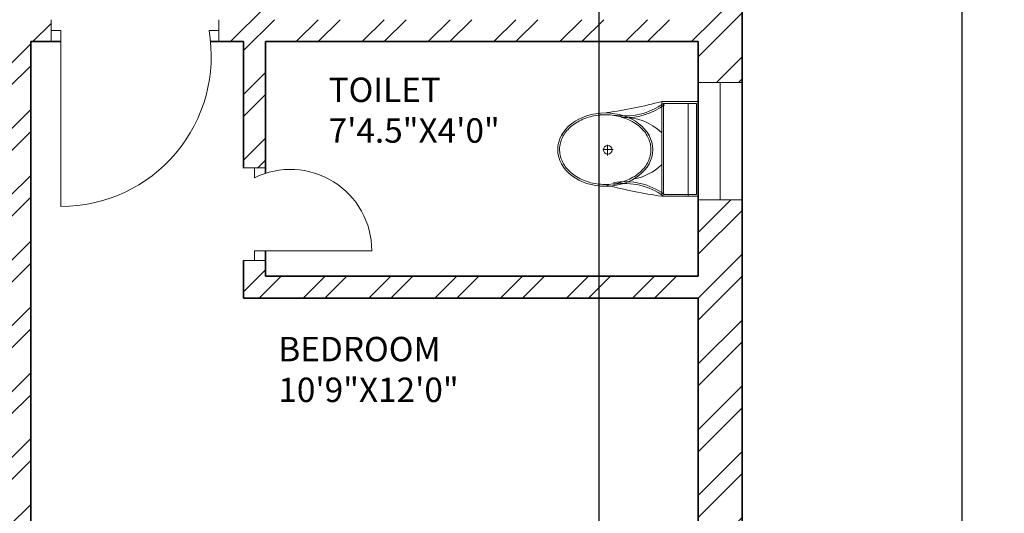
# Model space of a CAD drawing. Units: inches. Extents: x 2120 to 4013, y 1390 to 3019.
# Tile 22 of 59: x 2862 to 3063, y 1690 to 1792. Entities that reach past the tile are written whole.
import ezdxf

# ---------------------------------------------------------------- set-up
doc = ezdxf.new("R2010")
doc.units = ezdxf.units.IN
for name, color, linetype, lineweight in [('A-ANNO-DIMS', 2, 'Continuous', 18), ('A-AREA-IDEN', 7, 'Continuous', 18), ('A-DOOR', 3, 'Continuous', 18), ('A-FLOR-FIXT', 9, 'Continuous', 18), ('A-GLAZ', 4, 'Continuous', 18), ('A-WALL', 7, 'Continuous', 35), ('A-WALL-PATT', 252, 'Continuous', 13)]:
    doc.layers.add(name, color=color, linetype=linetype, lineweight=lineweight)
doc.styles.get("Standard").update_dxf_attribs({"font": 'arial.ttf'})
doc.dimstyles.get("Standard").update_dxf_attribs({"dimtxt": 0.18, "dimasz": 0.18, "dimexe": 0.18, "dimexo": 0.0625, "dimgap": 0.09, "dimtad": 0, "dimtih": 1, "dimtoh": 1, "dimdec": 4, "dimzin": 0, "dimdsep": 46, "dimtxsty": 'Standard', "dimcen": 0.09, "dimadec": 0, "dimazin": 0, "dimtfac": 1, "dimtdec": 4, "dimtofl": 0, "dimtmove": 0, "dimatfit": 3, "dimfxl": 1, "dimtolj": 1, "dimtzin": 0, "dimarcsym": 0})

# ---------------------------------------------------------------- blocks, each defined once
blk = doc.blocks.new('A$C31115884')
for p, q in [((283.1, 497.7), (223.4, 497.7)), ((257.5, 466.4), (257.5, 523.2)), ((0, 200), (0, 0)), ((520, 200), (0, 200)), ((10, 190), (10, 10)), ((510, 190), (10, 190)), ((510, 10), (510, 190)), ((520, 0), (520, 200)), ((510, 54.5), (0, 54.5)), ((10, 10), (510, 10)), ((0, 0), (520, 0))]:
    blk.add_line(p, q)
blk.add_circle((255.6, 496.4), 23.6)
for centre, radius, start, end in [((2777.7, -204.6), 2807, 165.4549, 171.7133), ((3237, 905), 2807, 188.2867, 194.5451), ((-294.5, 403.3), 364.7, 324.2091, 9.3499), ((-294.5, 403.3), 374.7, 324.2091, 9.3499), ((805.8, 403.3), 364.7, 170.6501, 215.7909), ((139.5, 406.2), 293.5, 315.8436, 2.6563), ((805.8, 403.3), 374.7, 179.2036, 215.7909), ((383.6, 406.2), 293.5, 190.2774, 224.1564)]:
    blk.add_arc(centre, radius, start, end)
blk.add_ellipse((256.2, 509.9), major_axis=(0, -260.7), ratio=0.772727)
blk.add_open_spline([(256.2, 259.2), (263.1, 259.2), (270, 259.7), (287.8, 262.3), (298.7, 265.1), (319.9, 273.1), (330.2, 278.4), (350.1, 291.1), (359.7, 298.7), (377.7, 315.9), (386.2, 325.5), (401.7, 346.6), (408.8, 358.1), (421.3, 382.5), (426.8, 395.5), (435.9, 422.4), (439.5, 436.4), (444.8, 465.1), (446.5, 479.7), (447.9, 509.2), (447.6, 524), (445, 553.3), (442.7, 567.8), (436.3, 596), (432.1, 609.7), (421.9, 636), (416, 648.6), (402.5, 672.1), (395, 683), (378.6, 703), (369.8, 712.1), (351.1, 728), (341.3, 734.8), (320.9, 746.2), (310.4, 750.7), (288.9, 757.3), (278, 759.4), (256, 761), (245, 760.6), (223.1, 757.2), (212.3, 754.3), (191.1, 746.1), (180.8, 740.7), (160.9, 727.8), (151.4, 720.1), (133.5, 702.7), (125.1, 693), (109.6, 671.7), (102.6, 660.2), (90.2, 635.7), (84.9, 622.7), (76, 595.6), (72.4, 581.6), (67.2, 552.9), (65.6, 538.2), (64.4, 508.8), (64.8, 494), (67.5, 464.7), (69.9, 450.2), (76.6, 422), (80.8, 408.3), (91.1, 382.2), (97.2, 369.7), (110.8, 346.3), (118.4, 335.4), (134.8, 315.6), (143.7, 306.7), (162.4, 290.9), (172.3, 284.2), (192.8, 273), (203.3, 268.6), (224.8, 262.2), (235.8, 260.2), (249.9, 259.3), (253, 259.2), (256.2, 259.2)], degree=3, knots=[0, 0, 0, 0, 0.110105, 0.110105, 0.285049, 0.285049, 0.459994, 0.459994, 0.634938, 0.634938, 0.809882, 0.809882, 0.984827, 0.984827, 1.159771, 1.159771, 1.334715, 1.334715, 1.50966, 1.50966, 1.684604, 1.684604, 1.859549, 1.859549, 2.034493, 2.034493, 2.209437, 2.209437, 2.384382, 2.384382, 2.559326, 2.559326, 2.73427, 2.73427, 2.909215, 2.909215, 3.084159, 3.084159, 3.259103, 3.259103, 3.434048, 3.434048, 3.608992, 3.608992, 3.783936, 3.783936, 3.958881, 3.958881, 4.133825, 4.133825, 4.30877, 4.30877, 4.483714, 4.483714, 4.658658, 4.658658, 4.833603, 4.833603, 5.008547, 5.008547, 5.183491, 5.183491, 5.358436, 5.358436, 5.53338, 5.53338, 5.708324, 5.708324, 5.883269, 5.883269, 6.058213, 6.058213, 6.233158, 6.233158, 6.283185, 6.283185, 6.283185, 6.283185])
blk = doc.blocks.new('DOOR-SWING-24IN-116p21DEG')
for p, q in [((0, 18.94), (4.5, 18.94)), ((4.5, 18.94), (2.25, 18.94)), ((2.25, 18.94), (2.25, 16.94)), ((4.5, 0), (0, 0)), ((0, 0), (2.25, 0)), ((2.25, 0), (2.25, 2)), ((2.25, 2), (26.25, 2))]:
    blk.add_line(p, q)
blk.add_arc((9.6, 2), 16.65, 0, 116.2087)
blk = doc.blocks.new('DOOR-SWING-36IN-99p84DEG')
for p, q in [((0, 38.25), (0, 33.75)), ((0, 33.75), (0, 38.25)), ((0, 38.25), (0, 36)), ((34.3, 38.25), (34.3, 33.75)), ((0, 36), (2, 36)), ((2, 36), (2, 0)), ((34.3, 36), (32.3, 36)), ((34.3, 33.75), (34.3, 36))]:
    blk.add_line(p, q)
blk.add_arc((2, 30.75), 30.75, 270, 9.8355)
blk = doc.blocks.new('WIN-PLAN-24IN-03')
for p, q in [((9, 24), (0, 24)), ((0, 24), (4.5, 24)), ((4.5, 24), (4.5, 0)), ((9, 0), (0, 0)), ((4.5, 0), (9, 0))]:
    blk.add_line(p, q)
blk = doc.blocks.new('*D212')
at = {"layer": 'A-ANNO-DIMS', "color": 0, "lineweight": -2, "transparency": 16777216}
for p, q in [((3009.8, 2352.53), (3054.91, 2352.53)), ((3054.73, 2352.35), (3054.73, 1947.71)), ((3054.73, 1542.71), (3054.73, 1947.35)), ((3009.8, 1542.53), (3054.91, 1542.53))]:
    blk.add_line(p, q, dxfattribs=at)
at = {"layer": 'A-ANNO-DIMS', "color": 0, "transparency": 16777216}
for points in [[(3054.7, 2352.35), (3054.76, 2352.35), (3054.73, 2352.53)], [(3054.7, 1542.71), (3054.76, 1542.71), (3054.73, 1542.53)]]:
    blk.add_solid(points, dxfattribs=at)
at = {"layer": 'Defpoints', "color": 0, "transparency": 16777216}
for p in [(3009.73, 2352.53), (3009.73, 1542.53), (3054.73, 1542.53)]:
    blk.add_point(p, dxfattribs=at)
at = {"layer": 'A-ANNO-DIMS', "color": 0, "transparency": 16777216, "insert": (3054.73, 1947.53), "char_height": 0.18, "attachment_point": 5}
blk.add_mtext('\\A1;810', dxfattribs=at)
blk = doc.blocks.new('*D217')
at = {"layer": 'A-ANNO-DIMS', "color": 0, "lineweight": -2, "transparency": 16777216}
for p, q in [((3071.67, 2352.53), (2980.31, 2352.53)), ((2980.49, 2352.35), (2980.49, 1947.71)), ((2980.49, 1542.71), (2980.49, 1947.35)), ((3305.67, 1542.53), (2980.31, 1542.53))]:
    blk.add_line(p, q, dxfattribs=at)
at = {"layer": 'A-ANNO-DIMS', "color": 0, "transparency": 16777216}
for points in [[(2980.46, 2352.35), (2980.52, 2352.35), (2980.49, 2352.53)], [(2980.46, 1542.71), (2980.52, 1542.71), (2980.49, 1542.53)]]:
    blk.add_solid(points, dxfattribs=at)
at = {"layer": 'Defpoints', "color": 0, "transparency": 16777216}
for p in [(2980.49, 2352.53), (3071.73, 2352.53), (3305.73, 1542.53)]:
    blk.add_point(p, dxfattribs=at)
at = {"layer": 'A-ANNO-DIMS', "color": 0, "transparency": 16777216, "insert": (2980.49, 1947.53), "char_height": 0.18, "attachment_point": 5}
blk.add_mtext('\\A1;810', dxfattribs=at)

msp = doc.modelspace()

# ---------------------------------------------------------------- hatches: boundary and pattern name
at = {"layer": 'A-WALL-PATT'}
h = msp.add_hatch(dxfattribs=at)
h.set_pattern_fill('ANSI32', color=256)
h.paths.add_polyline_path([(2271.7331, 2343.531), (2283.3788, 2343.531), (2283.3788, 2348.031), (2283.3788, 2352.5306), (2262.7331, 2352.5306), (2262.7331, 2182.638), (2267.2331, 2182.638), (2271.7331, 2182.638), (2271.7331, 2219.031), (2391.7331, 2219.031), (2391.7331, 2214.189), (2393.9831, 2214.189), (2396.2331, 2214.189), (2396.2331, 2219.031), (2420.2331, 2219.031), (2420.2331, 2225.7535), (2417.2197, 2225.7535), (2415.7331, 2225.7535), (2415.7331, 2223.5306), (2271.7331, 2223.5306)])
h.paths.add_polyline_path([(2380.0942, 2352.5306), (2343.3788, 2352.5306), (2343.3788, 2343.531), (2363.2331, 2343.531), (2363.2331, 2288.8489), (2365.4831, 2288.8489), (2367.7331, 2288.8489), (2367.7331, 2343.531), (2380.0942, 2343.531)], flags=17)
h.paths.add_polyline_path([(2432.4339, 2352.5306), (2404.0943, 2352.5306), (2404.0943, 2343.531), (2415.7331, 2343.531), (2415.7331, 2264.0306), (2367.7331, 2264.0306), (2367.7331, 2266.4872), (2363.2331, 2266.4872), (2363.2331, 2259.531), (2367.7331, 2259.531), (2415.7331, 2259.531), (2415.7331, 2255.0658), (2420.2331, 2255.0658), (2420.2331, 2259.531), (2424.5717, 2259.531), (2424.5717, 2261.781), (2424.5717, 2264.0306), (2420.2331, 2264.0306), (2420.2331, 2343.531), (2432.4339, 2343.531)])
h.paths.add_polyline_path([(2508.9115, 2352.5306), (2456.4339, 2352.5306), (2456.4339, 2343.531), (2468.2331, 2343.531), (2468.2331, 2264.0306), (2448.0487, 2264.0306), (2448.0487, 2259.531), (2468.2331, 2259.531), (2468.2331, 2255.5496), (2472.7331, 2255.5496), (2472.7331, 2343.531), (2508.9115, 2343.531)])
h.paths.add_polyline_path([(2637.7331, 2352.5306), (2544.9116, 2352.5306), (2544.9116, 2343.531), (2589.7331, 2343.531), (2633.2331, 2343.531), (2637.7331, 2343.531)])
h.paths.add_polyline_path([(2594.2331, 2343.5306), (2589.7331, 2343.5306), (2589.7331, 2259.5306), (2589.7331, 2252.4915), (2591.9831, 2252.4915), (2594.2331, 2252.4915)])
h.paths.add_polyline_path([(2637.7331, 2223.5306), (2594.2331, 2223.5306), (2594.2331, 2230.1988), (2591.9831, 2230.1988), (2589.7331, 2230.1988), (2589.7331, 2223.5306), (2472.7331, 2223.5306), (2468.2331, 2223.5306), (2468.2331, 2219.031), (2628.7331, 2219.031), (2628.7331, 2138.031), (2637.7331, 2138.031)])
h.paths.add_polyline_path([(3822.6535, 2458.4402), (3874.9468, 2458.4402), (3874.9468, 2476.9866), (3822.6535, 2476.9866)], flags=9)
h.paths.add_polyline_path([(3834.6921, 2781.8174), (3935.9206, 2781.8174), (3935.9206, 2800.3638), (3834.6921, 2800.3638)], flags=9)
h.paths.add_polyline_path([(3832.2843, 2837.9683), (3884.5776, 2837.9683), (3884.5776, 2856.5146), (3832.2843, 2856.5146)], flags=9)
h.paths.add_polyline_path([(3830.9388, 2861.4782), (3956.8958, 2861.4782), (3956.8958, 2880.0245), (3830.9388, 2880.0245)], flags=9)
h.paths.add_polyline_path([(3870.6966, 2352.5752), (3887.9272, 2352.5752), (3887.9272, 2377.3037), (3870.6966, 2377.3037)], flags=9)
h.paths.add_polyline_path([(3289.2701, 2413.161), (3435.2223, 2413.161), (3435.2223, 2450.2538), (3289.2701, 2450.2538)], flags=9)
h.paths.add_polyline_path([(2487.6944, 2414.3601), (2637.8335, 2414.3601), (2637.8335, 2451.4528), (2487.6944, 2451.4528)], flags=9)
h.paths.add_polyline_path([(2567.3724, 1457.9199), (2815.296, 1457.9199), (2815.296, 1495.0127), (2567.3724, 1495.0127)], flags=9)
h.paths.add_polyline_path([(2655.3825, 2093.2363), (2685.9555, 2093.2363), (2685.9555, 2111.8937), (2655.3825, 2111.8937)], flags=9)
h.paths.add_polyline_path([(2543.9218, 1550.6671), (2587.8406, 1550.6671), (2587.8406, 1569.3244), (2543.9218, 1569.3244)], flags=9)
h.paths.add_polyline_path([(2905.1384, 1543.8113), (2949.0572, 1543.8113), (2949.0572, 1562.4686), (2905.1384, 1562.4686)], flags=9)
h.paths.add_polyline_path([(2736.4118, 1702.4736), (2784.2153, 1702.4736), (2784.2153, 1721.1309), (2736.4118, 1721.1309)], flags=9)
h.paths.add_polyline_path([(2912.8666, 1710.4168), (2951.707, 1710.4168), (2951.707, 1729.0741), (2912.8666, 1729.0741)], flags=9)
h.paths.add_polyline_path([(2923.5785, 1763.5038), (2959.7279, 1763.5038), (2959.7279, 1782.1611), (2923.5785, 1782.1611)], flags=9)
h.paths.add_polyline_path([(2925.2114, 1809.6137), (2967.1861, 1809.6137), (2967.1861, 1828.271), (2925.2114, 1828.271)], flags=9)
h.paths.add_polyline_path([(2996.2711, 1878.9003), (2996.2711, 1913.109), (2977.6138, 1913.109), (2977.6138, 1878.9003)], flags=9)
h.paths.add_polyline_path([(2883.0859, 1895.7192), (2927.1855, 1895.7192), (2927.1855, 1914.3766), (2883.0859, 1914.3766)], flags=9)
h.paths.add_polyline_path([(2787.3924, 1810.8013), (2841.0213, 1810.8013), (2841.0213, 1829.4587), (2787.3924, 1829.4587)], flags=9)
h.paths.add_polyline_path([(2775.6399, 2101.7395), (2829.2689, 2101.7395), (2829.2689, 2120.3968), (2775.6399, 2120.3968)], flags=9)
h.paths.add_polyline_path([(2913.0263, 2075.817), (2951.8667, 2075.817), (2951.8667, 2094.4744), (2913.0263, 2094.4744)], flags=9)
h.paths.add_polyline_path([(2929.966, 2133.3669), (2966.1154, 2133.3669), (2966.1154, 2152.0243), (2929.966, 2152.0243)], flags=9)
h.paths.add_polyline_path([(2932.7502, 2182.6088), (2968.8996, 2182.6088), (2968.8996, 2201.2662), (2932.7502, 2201.2662)], flags=9)
h.paths.add_polyline_path([(2996.0681, 2266.3173), (2996.0681, 2300.5261), (2977.4108, 2300.5261), (2977.4108, 2266.3173)], flags=9)
h.paths.add_polyline_path([(2885.1039, 2279.2186), (2929.2035, 2279.2186), (2929.2035, 2297.8759), (2885.1039, 2297.8759)], flags=9)
h.paths.add_polyline_path([(2735.7042, 2218.3197), (2783.5078, 2218.3197), (2783.5078, 2236.9771), (2735.7042, 2236.9771)], flags=9)
h.paths.add_polyline_path([(2635.6049, 2044.0085), (2648.9678, 2044.0085), (2648.9678, 2054.312), (2635.6049, 2054.312)], flags=9)
h.paths.add_polyline_path([(2714.0148, 1923.0473), (2727.3777, 1923.0473), (2727.3777, 1933.3508), (2714.0148, 1933.3508)], flags=9)
h.paths.add_polyline_path([(2709.0345, 1988.1628), (2722.3974, 1988.1628), (2722.3974, 1998.4663), (2709.0345, 1998.4663)], flags=9)
h.paths.add_polyline_path([(2592.8935, 1962.1763), (2606.2564, 1962.1763), (2606.2564, 1972.4799), (2592.8935, 1972.4799)], flags=9)
h.paths.add_polyline_path([(2618.3996, 1985.9724), (2644.1942, 1985.9724), (2644.1942, 1996.2759), (2618.3996, 1996.2759)], flags=9)
h.paths.add_polyline_path([(2601.279, 1920.5869), (2614.6419, 1920.5869), (2614.6419, 1930.8904), (2601.279, 1930.8904)], flags=9)
h.paths.add_polyline_path([(2692.3278, 1932.7645), (2704.5311, 1932.7645), (2704.5311, 1943.0681), (2692.3278, 1943.0681)], flags=9)
h.paths.add_polyline_path([(2311.122, 1672.7318), (2355.0408, 1672.7318), (2355.0408, 1691.3892), (2311.122, 1691.3892)], flags=9)
h.paths.add_polyline_path([(2456.2551, 1632.3198), (2492.4796, 1632.3198), (2492.4796, 1650.9772), (2456.2551, 1650.9772)], flags=9)
h.paths.add_polyline_path([(2401.0766, 1631.4793), (2437.301, 1631.4793), (2437.301, 1650.1367), (2401.0766, 1650.1367)], flags=9)
h.paths.add_polyline_path([(2546.7054, 1700.9235), (2594.509, 1700.9235), (2594.509, 1719.5809), (2546.7054, 1719.5809)], flags=9)
h.paths.add_polyline_path([(2445.4866, 1766.9937), (2497.5261, 1766.9937), (2497.5261, 1785.651), (2445.4866, 1785.651)], flags=9)
h.paths.add_polyline_path([(2287.9992, 1739.7675), (2326.8396, 1739.7675), (2326.8396, 1758.4248), (2287.9992, 1758.4248)], flags=9)
h.paths.add_polyline_path([(2458.5279, 1924.7607), (2510.5675, 1924.7607), (2510.5675, 1943.4181), (2458.5279, 1943.4181)], flags=9)
h.paths.add_polyline_path([(2309.2811, 1902.7642), (2345.4305, 1902.7642), (2345.4305, 1921.4215), (2309.2811, 1921.4215)], flags=9)
h.paths.add_polyline_path([(2490.7554, 2018.9392), (2530.7896, 2018.9392), (2530.7896, 2037.5965), (2490.7554, 2037.5965)], flags=9)
h.paths.add_polyline_path([(2402.143, 2024.7393), (2438.5414, 2024.7393), (2438.5414, 2043.3966), (2402.143, 2043.3966)], flags=9)
h.paths.add_polyline_path([(2287.856, 1931.7926), (2326.6964, 1931.7926), (2326.6964, 1950.4499), (2287.856, 1950.4499)], flags=9)
h.paths.add_polyline_path([(2281.7979, 2193.5771), (2320.6383, 2193.5771), (2320.6383, 2212.2344), (2281.7979, 2212.2344)], flags=25)
h.paths.add_polyline_path([(2484.0754, 2093.892), (2536.115, 2093.892), (2536.115, 2112.5494), (2484.0754, 2112.5494)], flags=9)
h.paths.add_polyline_path([(2624.7948, 2281.8639), (2624.7948, 2311.4137), (2606.1375, 2311.4137), (2606.1375, 2281.8639)], flags=9)
h.paths.add_polyline_path([(2507.5036, 2290.3639), (2541.934, 2290.3639), (2541.934, 2309.0212), (2507.5036, 2309.0212)], flags=9)
h.paths.add_polyline_path([(2423.1076, 2285.2202), (2459.332, 2285.2202), (2459.332, 2303.8776), (2423.1076, 2303.8776)], flags=9)
h.paths.add_polyline_path([(2374.5467, 2289.6272), (2410.7711, 2289.6272), (2410.7711, 2308.2846), (2374.5467, 2308.2846)], flags=25)
h.paths.add_polyline_path([(2277.4907, 2227.5651), (2316.3311, 2227.5651), (2316.3311, 2246.2224), (2277.4907, 2246.2224)], flags=25)
h.paths.add_polyline_path([(2655.3825, 2093.2367), (2685.9555, 2093.2367), (2685.9555, 2111.894), (2655.3825, 2111.894)], flags=9)
h.paths.add_polyline_path([(2543.9217, 1550.6674), (2587.8406, 1550.6674), (2587.8406, 1569.3247), (2543.9217, 1569.3247)], flags=9)
h.paths.add_polyline_path([(2905.1384, 1543.8116), (2949.0572, 1543.8116), (2949.0572, 1562.4689), (2905.1384, 1562.4689)], flags=9)
h.paths.add_polyline_path([(2736.4118, 1702.4739), (2784.2153, 1702.4739), (2784.2153, 1721.1312), (2736.4118, 1721.1312)], flags=9)
h.paths.add_polyline_path([(2912.8666, 1710.4171), (2951.707, 1710.4171), (2951.707, 1729.0744), (2912.8666, 1729.0744)], flags=9)
h.paths.add_polyline_path([(2923.5785, 1763.5041), (2959.7279, 1763.5041), (2959.7279, 1782.1614), (2923.5785, 1782.1614)], flags=9)
h.paths.add_polyline_path([(2925.2114, 1809.614), (2967.1861, 1809.614), (2967.1861, 1828.2713), (2925.2114, 1828.2713)], flags=9)
h.paths.add_polyline_path([(2996.2711, 1878.9006), (2996.2711, 1913.1094), (2977.6137, 1913.1094), (2977.6137, 1878.9006)], flags=9)
h.paths.add_polyline_path([(2883.0859, 1895.7195), (2927.1855, 1895.7195), (2927.1855, 1914.3769), (2883.0859, 1914.3769)], flags=9)
h.paths.add_polyline_path([(2787.3924, 1810.8016), (2841.0213, 1810.8016), (2841.0213, 1829.459), (2787.3924, 1829.459)], flags=9)
h.paths.add_polyline_path([(2775.6399, 2101.7398), (2829.2688, 2101.7398), (2829.2688, 2120.3971), (2775.6399, 2120.3971)], flags=9)
h.paths.add_polyline_path([(2913.0263, 2075.8173), (2951.8667, 2075.8173), (2951.8667, 2094.4747), (2913.0263, 2094.4747)], flags=9)
h.paths.add_polyline_path([(2929.966, 2133.3672), (2966.1154, 2133.3672), (2966.1154, 2152.0246), (2929.966, 2152.0246)], flags=9)
h.paths.add_polyline_path([(2932.7502, 2182.6091), (2968.8996, 2182.6091), (2968.8996, 2201.2665), (2932.7502, 2201.2665)], flags=9)
h.paths.add_polyline_path([(2996.0681, 2266.3176), (2996.0681, 2300.5264), (2977.4108, 2300.5264), (2977.4108, 2266.3176)], flags=9)
h.paths.add_polyline_path([(2885.1039, 2279.2189), (2929.2035, 2279.2189), (2929.2035, 2297.8762), (2885.1039, 2297.8762)], flags=9)
h.paths.add_polyline_path([(2735.7042, 2218.32), (2783.5078, 2218.32), (2783.5078, 2236.9774), (2735.7042, 2236.9774)], flags=9)
h.paths.add_polyline_path([(2635.6048, 2044.0088), (2648.9677, 2044.0088), (2648.9677, 2054.3123), (2635.6048, 2054.3123)], flags=9)
h.paths.add_polyline_path([(2714.0148, 1923.0476), (2727.3777, 1923.0476), (2727.3777, 1933.3511), (2714.0148, 1933.3511)], flags=9)
h.paths.add_polyline_path([(2709.0345, 1988.1631), (2722.3974, 1988.1631), (2722.3974, 1998.4666), (2709.0345, 1998.4666)], flags=9)
h.paths.add_polyline_path([(2592.8935, 1962.1766), (2606.2564, 1962.1766), (2606.2564, 1972.4802), (2592.8935, 1972.4802)], flags=9)
h.paths.add_polyline_path([(2618.3995, 1985.9727), (2644.1942, 1985.9727), (2644.1942, 1996.2762), (2618.3995, 1996.2762)], flags=9)
h.paths.add_polyline_path([(2601.279, 1920.5872), (2614.6419, 1920.5872), (2614.6419, 1930.8908), (2601.279, 1930.8908)], flags=9)
h.paths.add_polyline_path([(2692.3278, 1932.7648), (2704.5311, 1932.7648), (2704.5311, 1943.0684), (2692.3278, 1943.0684)], flags=9)
h.paths.add_polyline_path([(2311.122, 1672.7321), (2355.0408, 1672.7321), (2355.0408, 1691.3895), (2311.122, 1691.3895)], flags=9)
h.paths.add_polyline_path([(2456.2551, 1632.3201), (2492.4795, 1632.3201), (2492.4795, 1650.9775), (2456.2551, 1650.9775)], flags=9)
h.paths.add_polyline_path([(2401.0766, 1631.4796), (2437.301, 1631.4796), (2437.301, 1650.137), (2401.0766, 1650.137)], flags=9)
h.paths.add_polyline_path([(2546.7054, 1700.9238), (2594.509, 1700.9238), (2594.509, 1719.5812), (2546.7054, 1719.5812)], flags=9)
h.paths.add_polyline_path([(2445.4866, 1766.994), (2497.5261, 1766.994), (2497.5261, 1785.6513), (2445.4866, 1785.6513)], flags=9)
h.paths.add_polyline_path([(2287.9992, 1739.7678), (2326.8396, 1739.7678), (2326.8396, 1758.4251), (2287.9992, 1758.4251)], flags=9)
h.paths.add_polyline_path([(2458.5279, 1924.7611), (2510.5675, 1924.7611), (2510.5675, 1943.4184), (2458.5279, 1943.4184)], flags=9)
h.paths.add_polyline_path([(2309.2811, 1902.7645), (2345.4305, 1902.7645), (2345.4305, 1921.4218), (2309.2811, 1921.4218)], flags=9)
h.paths.add_polyline_path([(2490.7554, 2018.9395), (2530.7895, 2018.9395), (2530.7895, 2037.5968), (2490.7554, 2037.5968)], flags=9)
h.paths.add_polyline_path([(2402.143, 2024.7396), (2438.5413, 2024.7396), (2438.5413, 2043.3969), (2402.143, 2043.3969)], flags=9)
h.paths.add_polyline_path([(2287.856, 1931.7929), (2326.6964, 1931.7929), (2326.6964, 1950.4502), (2287.856, 1950.4502)], flags=9)
h.paths.add_polyline_path([(2281.7979, 2193.5774), (2320.6383, 2193.5774), (2320.6383, 2212.2347), (2281.7979, 2212.2347)], flags=25)
h.paths.add_polyline_path([(2484.0754, 2093.8924), (2536.115, 2093.8924), (2536.115, 2112.5497), (2484.0754, 2112.5497)], flags=9)
h.paths.add_polyline_path([(2624.7948, 2281.8642), (2624.7948, 2311.414), (2606.1374, 2311.414), (2606.1374, 2281.8642)], flags=9)
h.paths.add_polyline_path([(2507.5035, 2290.3642), (2541.934, 2290.3642), (2541.934, 2309.0215), (2507.5035, 2309.0215)], flags=9)
h.paths.add_polyline_path([(2423.1075, 2285.2205), (2459.332, 2285.2205), (2459.332, 2303.8779), (2423.1075, 2303.8779)], flags=9)
h.paths.add_polyline_path([(2374.5467, 2289.6275), (2410.7711, 2289.6275), (2410.7711, 2308.2849), (2374.5467, 2308.2849)], flags=25)
h.paths.add_polyline_path([(2277.4907, 2227.5654), (2316.3311, 2227.5654), (2316.3311, 2246.2227), (2277.4907, 2246.2227)], flags=25)
h = msp.add_hatch(dxfattribs=at)
h.set_pattern_fill('ANSI32', color=256)
h.paths.add_polyline_path([(2271.7331, 1980.389), (2262.7331, 1980.389), (2262.7331, 1912.8434), (2267.2331, 1912.8434), (2271.7331, 1912.8434), (2271.7331, 1922.531), (2351.2331, 1922.531), (2351.2331, 1901.4728), (2355.7331, 1901.4728), (2355.7331, 1922.531), (2357.9815, 1922.531), (2357.9815, 1926.5306), (2271.7331, 1926.5306)])
h.paths.add_polyline_path([(2589.2331, 1949.1622), (2584.7331, 1949.1622), (2580.2331, 1949.1622), (2580.2331, 1874.5306), (2355.7331, 1874.5306), (2355.7331, 1880.1922), (2351.2331, 1880.1922), (2351.2331, 1874.5306), (2271.7331, 1874.5306), (2271.7331, 1888.8431), (2262.7331, 1888.8431), (2262.7331, 1842.2909), (2267.2331, 1842.2909), (2271.7331, 1842.2909), (2271.7331, 1865.531), (2415.7331, 1865.531), (2415.7331, 1779.7286), (2420.2331, 1779.7286), (2420.2331, 1865.531), (2589.2331, 1865.531)])
h.paths.add_polyline_path([(2271.7331, 1782.2906), (2262.7331, 1782.2906), (2262.7331, 1711.4639), (2267.2331, 1711.4639), (2271.7331, 1711.4639), (2271.7331, 1738.031), (2420.2331, 1738.031), (2420.2331, 1742.531), (2420.2331, 1747.3376), (2417.9831, 1747.3376), (2415.7331, 1747.3376), (2415.7331, 1742.5306), (2271.7331, 1742.5306)])
h.paths.add_polyline_path([(2271.7331, 1627.031), (2362.3957, 1627.031), (2362.3957, 1629.281), (2362.3957, 1631.5306), (2271.7331, 1631.5306), (2271.7331, 1675.4636), (2262.7331, 1675.4636), (2262.7331, 1581.531), (2405.3032, 1581.531), (2405.3032, 1586.031), (2405.3032, 1590.5306), (2396.2331, 1590.5306), (2396.2331, 1691.4513), (2418.7206, 1691.4513), (2418.7206, 1695.951), (2396.2331, 1695.951), (2391.7331, 1695.951), (2391.7331, 1631.5306), (2386.7425, 1631.5306), (2386.7425, 1629.2806), (2386.7425, 1627.031), (2391.7331, 1627.031), (2391.7331, 1586.1709), (2271.7331, 1586.1709)])
h.paths.add_polyline_path([(2459.6703, 1590.5306), (2429.3032, 1590.5306), (2429.3032, 1581.531), (2459.6703, 1581.531), (2459.6703, 1586.031)])
h.paths.add_polyline_path([(2501.2331, 1590.531), (2501.2331, 1665.0195), (2498.9831, 1665.0195), (2496.7331, 1665.0195), (2496.7331, 1590.5306), (2483.8201, 1590.5306), (2483.8201, 1590.1579), (2483.6704, 1590.1579), (2483.6704, 1581.531), (2505.0196, 1581.531), (2505.0196, 1583.781), (2505.0196, 1586.0306), (2501.2331, 1586.0306)])
h.paths.add_polyline_path([(2544.1361, 1583.781), (2544.1361, 1586.0306), (2527.1368, 1586.0306), (2527.1368, 1583.7806), (2527.1368, 1581.531), (2544.1361, 1581.531)])
h.paths.add_polyline_path([(3822.6535, 2458.4402), (3874.9468, 2458.4402), (3874.9468, 2476.9866), (3822.6535, 2476.9866)], flags=9)
h.paths.add_polyline_path([(3834.6921, 2781.8174), (3935.9206, 2781.8174), (3935.9206, 2800.3638), (3834.6921, 2800.3638)], flags=9)
h.paths.add_polyline_path([(3832.2843, 2837.9683), (3884.5776, 2837.9683), (3884.5776, 2856.5146), (3832.2843, 2856.5146)], flags=9)
h.paths.add_polyline_path([(3830.9388, 2861.4782), (3956.8958, 2861.4782), (3956.8958, 2880.0245), (3830.9388, 2880.0245)], flags=9)
h.paths.add_polyline_path([(3870.6966, 2352.5752), (3887.9272, 2352.5752), (3887.9272, 2377.3037), (3870.6966, 2377.3037)], flags=9)
h.paths.add_polyline_path([(3289.2701, 2413.161), (3435.2223, 2413.161), (3435.2223, 2450.2538), (3289.2701, 2450.2538)], flags=9)
h.paths.add_polyline_path([(2487.6944, 2414.3601), (2637.8335, 2414.3601), (2637.8335, 2451.4528), (2487.6944, 2451.4528)], flags=9)
h.paths.add_polyline_path([(2567.3724, 1457.9199), (2815.296, 1457.9199), (2815.296, 1495.0127), (2567.3724, 1495.0127)], flags=9)
h.paths.add_polyline_path([(2655.3825, 2093.2363), (2685.9555, 2093.2363), (2685.9555, 2111.8937), (2655.3825, 2111.8937)], flags=9)
h.paths.add_polyline_path([(2543.9218, 1550.6671), (2587.8406, 1550.6671), (2587.8406, 1569.3244), (2543.9218, 1569.3244)], flags=9)
h.paths.add_polyline_path([(2905.1384, 1543.8113), (2949.0572, 1543.8113), (2949.0572, 1562.4686), (2905.1384, 1562.4686)], flags=9)
h.paths.add_polyline_path([(2736.4118, 1702.4736), (2784.2153, 1702.4736), (2784.2153, 1721.1309), (2736.4118, 1721.1309)], flags=9)
h.paths.add_polyline_path([(2912.8666, 1710.4168), (2951.707, 1710.4168), (2951.707, 1729.0741), (2912.8666, 1729.0741)], flags=9)
h.paths.add_polyline_path([(2923.5785, 1763.5038), (2959.7279, 1763.5038), (2959.7279, 1782.1611), (2923.5785, 1782.1611)], flags=9)
h.paths.add_polyline_path([(2925.2114, 1809.6137), (2967.1861, 1809.6137), (2967.1861, 1828.271), (2925.2114, 1828.271)], flags=9)
h.paths.add_polyline_path([(2996.2711, 1878.9003), (2996.2711, 1913.109), (2977.6138, 1913.109), (2977.6138, 1878.9003)], flags=9)
h.paths.add_polyline_path([(2883.0859, 1895.7192), (2927.1855, 1895.7192), (2927.1855, 1914.3766), (2883.0859, 1914.3766)], flags=9)
h.paths.add_polyline_path([(2787.3924, 1810.8013), (2841.0213, 1810.8013), (2841.0213, 1829.4587), (2787.3924, 1829.4587)], flags=9)
h.paths.add_polyline_path([(2775.6399, 2101.7395), (2829.2689, 2101.7395), (2829.2689, 2120.3968), (2775.6399, 2120.3968)], flags=9)
h.paths.add_polyline_path([(2913.0263, 2075.817), (2951.8667, 2075.817), (2951.8667, 2094.4744), (2913.0263, 2094.4744)], flags=9)
h.paths.add_polyline_path([(2929.966, 2133.3669), (2966.1154, 2133.3669), (2966.1154, 2152.0243), (2929.966, 2152.0243)], flags=9)
h.paths.add_polyline_path([(2932.7502, 2182.6088), (2968.8996, 2182.6088), (2968.8996, 2201.2662), (2932.7502, 2201.2662)], flags=9)
h.paths.add_polyline_path([(2996.0681, 2266.3173), (2996.0681, 2300.5261), (2977.4108, 2300.5261), (2977.4108, 2266.3173)], flags=9)
h.paths.add_polyline_path([(2885.1039, 2279.2186), (2929.2035, 2279.2186), (2929.2035, 2297.8759), (2885.1039, 2297.8759)], flags=9)
h.paths.add_polyline_path([(2735.7042, 2218.3197), (2783.5078, 2218.3197), (2783.5078, 2236.9771), (2735.7042, 2236.9771)], flags=9)
h.paths.add_polyline_path([(2635.6049, 2044.0085), (2648.9678, 2044.0085), (2648.9678, 2054.312), (2635.6049, 2054.312)], flags=9)
h.paths.add_polyline_path([(2714.0148, 1923.0473), (2727.3777, 1923.0473), (2727.3777, 1933.3508), (2714.0148, 1933.3508)], flags=9)
h.paths.add_polyline_path([(2709.0345, 1988.1628), (2722.3974, 1988.1628), (2722.3974, 1998.4663), (2709.0345, 1998.4663)], flags=9)
h.paths.add_polyline_path([(2592.8935, 1962.1763), (2606.2564, 1962.1763), (2606.2564, 1972.4799), (2592.8935, 1972.4799)], flags=9)
h.paths.add_polyline_path([(2618.3996, 1985.9724), (2644.1942, 1985.9724), (2644.1942, 1996.2759), (2618.3996, 1996.2759)], flags=9)
h.paths.add_polyline_path([(2601.279, 1920.5869), (2614.6419, 1920.5869), (2614.6419, 1930.8904), (2601.279, 1930.8904)], flags=9)
h.paths.add_polyline_path([(2692.3278, 1932.7645), (2704.5311, 1932.7645), (2704.5311, 1943.0681), (2692.3278, 1943.0681)], flags=9)
h.paths.add_polyline_path([(2311.122, 1672.7318), (2355.0408, 1672.7318), (2355.0408, 1691.3892), (2311.122, 1691.3892)], flags=25)
h.paths.add_polyline_path([(2456.2551, 1632.3198), (2492.4796, 1632.3198), (2492.4796, 1650.9772), (2456.2551, 1650.9772)], flags=9)
h.paths.add_polyline_path([(2401.0766, 1631.4793), (2437.301, 1631.4793), (2437.301, 1650.1367), (2401.0766, 1650.1367)], flags=9)
h.paths.add_polyline_path([(2546.7054, 1700.9235), (2594.509, 1700.9235), (2594.509, 1719.5809), (2546.7054, 1719.5809)], flags=9)
h.paths.add_polyline_path([(2445.4866, 1766.9937), (2497.5261, 1766.9937), (2497.5261, 1785.651), (2445.4866, 1785.651)], flags=9)
h.paths.add_polyline_path([(2287.9992, 1739.7675), (2326.8396, 1739.7675), (2326.8396, 1758.4248), (2287.9992, 1758.4248)], flags=24)
h.paths.add_polyline_path([(2458.5279, 1924.7607), (2510.5675, 1924.7607), (2510.5675, 1943.4181), (2458.5279, 1943.4181)], flags=25)
h.paths.add_polyline_path([(2309.2811, 1902.7642), (2345.4305, 1902.7642), (2345.4305, 1921.4215), (2309.2811, 1921.4215)], flags=25)
h.paths.add_polyline_path([(2490.7554, 2018.9392), (2530.7896, 2018.9392), (2530.7896, 2037.5965), (2490.7554, 2037.5965)], flags=9)
h.paths.add_polyline_path([(2402.143, 2024.7393), (2438.5414, 2024.7393), (2438.5414, 2043.3966), (2402.143, 2043.3966)], flags=9)
h.paths.add_polyline_path([(2287.856, 1931.7926), (2326.6964, 1931.7926), (2326.6964, 1950.4499), (2287.856, 1950.4499)], flags=25)
h.paths.add_polyline_path([(2281.7979, 2193.5771), (2320.6383, 2193.5771), (2320.6383, 2212.2344), (2281.7979, 2212.2344)], flags=9)
h.paths.add_polyline_path([(2484.0754, 2093.892), (2536.115, 2093.892), (2536.115, 2112.5494), (2484.0754, 2112.5494)], flags=9)
h.paths.add_polyline_path([(2624.7948, 2281.8639), (2624.7948, 2311.4137), (2606.1375, 2311.4137), (2606.1375, 2281.8639)], flags=9)
h.paths.add_polyline_path([(2507.5036, 2290.3639), (2541.934, 2290.3639), (2541.934, 2309.0212), (2507.5036, 2309.0212)], flags=9)
h.paths.add_polyline_path([(2423.1076, 2285.2202), (2459.332, 2285.2202), (2459.332, 2303.8776), (2423.1076, 2303.8776)], flags=9)
h.paths.add_polyline_path([(2374.5467, 2289.6272), (2410.7711, 2289.6272), (2410.7711, 2308.2846), (2374.5467, 2308.2846)], flags=9)
h.paths.add_polyline_path([(2277.4907, 2227.5651), (2316.3311, 2227.5651), (2316.3311, 2246.2224), (2277.4907, 2246.2224)], flags=9)
h.paths.add_polyline_path([(2655.3825, 2093.2367), (2685.9555, 2093.2367), (2685.9555, 2111.894), (2655.3825, 2111.894)], flags=9)
h.paths.add_polyline_path([(2543.9217, 1550.6674), (2587.8406, 1550.6674), (2587.8406, 1569.3247), (2543.9217, 1569.3247)], flags=9)
h.paths.add_polyline_path([(2905.1384, 1543.8116), (2949.0572, 1543.8116), (2949.0572, 1562.4689), (2905.1384, 1562.4689)], flags=9)
h.paths.add_polyline_path([(2736.4118, 1702.4739), (2784.2153, 1702.4739), (2784.2153, 1721.1312), (2736.4118, 1721.1312)], flags=9)
h.paths.add_polyline_path([(2912.8666, 1710.4171), (2951.707, 1710.4171), (2951.707, 1729.0744), (2912.8666, 1729.0744)], flags=9)
h.paths.add_polyline_path([(2923.5785, 1763.5041), (2959.7279, 1763.5041), (2959.7279, 1782.1614), (2923.5785, 1782.1614)], flags=9)
h.paths.add_polyline_path([(2925.2114, 1809.614), (2967.1861, 1809.614), (2967.1861, 1828.2713), (2925.2114, 1828.2713)], flags=9)
h.paths.add_polyline_path([(2996.2711, 1878.9006), (2996.2711, 1913.1094), (2977.6137, 1913.1094), (2977.6137, 1878.9006)], flags=9)
h.paths.add_polyline_path([(2883.0859, 1895.7195), (2927.1855, 1895.7195), (2927.1855, 1914.3769), (2883.0859, 1914.3769)], flags=9)
h.paths.add_polyline_path([(2787.3924, 1810.8016), (2841.0213, 1810.8016), (2841.0213, 1829.459), (2787.3924, 1829.459)], flags=9)
h.paths.add_polyline_path([(2775.6399, 2101.7398), (2829.2688, 2101.7398), (2829.2688, 2120.3971), (2775.6399, 2120.3971)], flags=9)
h.paths.add_polyline_path([(2913.0263, 2075.8173), (2951.8667, 2075.8173), (2951.8667, 2094.4747), (2913.0263, 2094.4747)], flags=9)
h.paths.add_polyline_path([(2929.966, 2133.3672), (2966.1154, 2133.3672), (2966.1154, 2152.0246), (2929.966, 2152.0246)], flags=9)
h.paths.add_polyline_path([(2932.7502, 2182.6091), (2968.8996, 2182.6091), (2968.8996, 2201.2665), (2932.7502, 2201.2665)], flags=9)
h.paths.add_polyline_path([(2996.0681, 2266.3176), (2996.0681, 2300.5264), (2977.4108, 2300.5264), (2977.4108, 2266.3176)], flags=9)
h.paths.add_polyline_path([(2885.1039, 2279.2189), (2929.2035, 2279.2189), (2929.2035, 2297.8762), (2885.1039, 2297.8762)], flags=9)
h.paths.add_polyline_path([(2735.7042, 2218.32), (2783.5078, 2218.32), (2783.5078, 2236.9774), (2735.7042, 2236.9774)], flags=9)
h.paths.add_polyline_path([(2635.6048, 2044.0088), (2648.9677, 2044.0088), (2648.9677, 2054.3123), (2635.6048, 2054.3123)], flags=9)
h.paths.add_polyline_path([(2714.0148, 1923.0476), (2727.3777, 1923.0476), (2727.3777, 1933.3511), (2714.0148, 1933.3511)], flags=9)
h.paths.add_polyline_path([(2709.0345, 1988.1631), (2722.3974, 1988.1631), (2722.3974, 1998.4666), (2709.0345, 1998.4666)], flags=9)
h.paths.add_polyline_path([(2592.8935, 1962.1766), (2606.2564, 1962.1766), (2606.2564, 1972.4802), (2592.8935, 1972.4802)], flags=9)
h.paths.add_polyline_path([(2618.3995, 1985.9727), (2644.1942, 1985.9727), (2644.1942, 1996.2762), (2618.3995, 1996.2762)], flags=9)
h.paths.add_polyline_path([(2601.279, 1920.5872), (2614.6419, 1920.5872), (2614.6419, 1930.8908), (2601.279, 1930.8908)], flags=9)
h.paths.add_polyline_path([(2692.3278, 1932.7648), (2704.5311, 1932.7648), (2704.5311, 1943.0684), (2692.3278, 1943.0684)], flags=9)
h.paths.add_polyline_path([(2311.122, 1672.7321), (2355.0408, 1672.7321), (2355.0408, 1691.3895), (2311.122, 1691.3895)], flags=25)
h.paths.add_polyline_path([(2456.2551, 1632.3201), (2492.4795, 1632.3201), (2492.4795, 1650.9775), (2456.2551, 1650.9775)], flags=9)
h.paths.add_polyline_path([(2401.0766, 1631.4796), (2437.301, 1631.4796), (2437.301, 1650.137), (2401.0766, 1650.137)], flags=9)
h.paths.add_polyline_path([(2546.7054, 1700.9238), (2594.509, 1700.9238), (2594.509, 1719.5812), (2546.7054, 1719.5812)], flags=9)
h.paths.add_polyline_path([(2445.4866, 1766.994), (2497.5261, 1766.994), (2497.5261, 1785.6513), (2445.4866, 1785.6513)], flags=9)
h.paths.add_polyline_path([(2287.9992, 1739.7678), (2326.8396, 1739.7678), (2326.8396, 1758.4251), (2287.9992, 1758.4251)], flags=24)
h.paths.add_polyline_path([(2458.5279, 1924.7611), (2510.5675, 1924.7611), (2510.5675, 1943.4184), (2458.5279, 1943.4184)], flags=25)
h.paths.add_polyline_path([(2309.2811, 1902.7645), (2345.4305, 1902.7645), (2345.4305, 1921.4218), (2309.2811, 1921.4218)], flags=25)
h.paths.add_polyline_path([(2490.7554, 2018.9395), (2530.7895, 2018.9395), (2530.7895, 2037.5968), (2490.7554, 2037.5968)], flags=9)
h.paths.add_polyline_path([(2402.143, 2024.7396), (2438.5413, 2024.7396), (2438.5413, 2043.3969), (2402.143, 2043.3969)], flags=9)
h.paths.add_polyline_path([(2287.856, 1931.7929), (2326.6964, 1931.7929), (2326.6964, 1950.4502), (2287.856, 1950.4502)], flags=25)
h.paths.add_polyline_path([(2281.7979, 2193.5774), (2320.6383, 2193.5774), (2320.6383, 2212.2347), (2281.7979, 2212.2347)], flags=9)
h.paths.add_polyline_path([(2484.0754, 2093.8924), (2536.115, 2093.8924), (2536.115, 2112.5497), (2484.0754, 2112.5497)], flags=9)
h.paths.add_polyline_path([(2624.7948, 2281.8642), (2624.7948, 2311.414), (2606.1374, 2311.414), (2606.1374, 2281.8642)], flags=9)
h.paths.add_polyline_path([(2507.5035, 2290.3642), (2541.934, 2290.3642), (2541.934, 2309.0215), (2507.5035, 2309.0215)], flags=9)
h.paths.add_polyline_path([(2423.1075, 2285.2205), (2459.332, 2285.2205), (2459.332, 2303.8779), (2423.1075, 2303.8779)], flags=9)
h.paths.add_polyline_path([(2374.5467, 2289.6275), (2410.7711, 2289.6275), (2410.7711, 2308.2849), (2374.5467, 2308.2849)], flags=9)
h.paths.add_polyline_path([(2277.4907, 2227.5654), (2316.3311, 2227.5654), (2316.3311, 2246.2227), (2277.4907, 2246.2227)], flags=9)
h = msp.add_hatch(dxfattribs=at)
h.set_pattern_fill('ANSI32', color=256)
h.paths.add_polyline_path([(2271.7331, 2122.6377), (2262.7331, 2122.6377), (2262.7331, 2040.3893), (2267.2331, 2040.3893), (2271.7331, 2040.3893), (2271.7331, 2044.8856), (2271.7331, 2070.531), (2391.7331, 2070.531), (2391.7331, 1926.5306), (2388.3993, 1926.5306), (2388.3993, 1922.531), (2395.7331, 1922.531), (2395.7331, 1992.531), (2400.4511, 1992.531), (2400.4511, 1997.0306), (2395.7331, 1997.0306), (2395.7331, 2070.531), (2443.7331, 2070.531), (2443.7331, 2046.1368), (2448.2331, 2046.1368), (2448.2331, 2070.531), (2580.2331, 2070.531), (2580.2331, 1997.0306), (2492.9076, 1997.0306), (2492.9076, 1992.531), (2580.2331, 1992.531), (2580.2331, 1983.9368), (2589.2331, 1983.9368), (2589.2331, 2070.531), (2589.2331, 2075.0306), (2396.2331, 2075.0306), (2396.2331, 2184.3565), (2393.9831, 2184.3565), (2391.7331, 2184.3565), (2391.7331, 2075.0306), (2271.7331, 2075.0306)])
h.paths.add_polyline_path([(2724.7331, 2138.0306), (2628.7331, 2138.0306), (2628.7331, 2070.5306), (2628.7331, 2067.0987), (2633.2331, 2067.0987), (2637.7331, 2067.0987), (2637.7331, 2070.531), (2657.3413, 2070.531), (2657.3413, 2079.5306), (2637.7331, 2079.5306), (2637.7331, 2129.031), (2715.7331, 2129.031), (2715.7331, 2079.5306), (2698.0378, 2079.5306), (2698.0378, 2070.531), (2715.7331, 2070.531), (2715.7331, 2012.1531), (2720.2331, 2012.1531), (2724.7331, 2012.1531)])
h.paths.add_polyline_path([(2724.7331, 2213.031), (2831.3209, 2213.031), (2831.3209, 2215.281), (2831.3209, 2217.5306), (2724.7331, 2217.5306), (2724.7331, 2343.531), (2751.8755, 2343.531), (2751.8755, 2352.5306), (2715.7331, 2352.5306), (2715.7331, 2138.031), (2724.7331, 2138.031)])
h.paths.add_polyline_path([(2902.53, 2352.5306), (2811.8755, 2352.5306), (2811.8755, 2343.531), (2867.2331, 2343.531), (2867.2331, 2217.5306), (2863.6364, 2217.5306), (2863.6364, 2213.031), (2871.7331, 2213.031), (2871.7331, 2217.531), (2871.7331, 2343.531), (2902.53, 2343.531)])
h.paths.add_polyline_path([(3009.7331, 2352.5306), (2938.53, 2352.5306), (2938.53, 2343.531), (2966.2331, 2343.531), (2966.2331, 2242.3281), (2968.4831, 2242.3281), (2970.7331, 2242.3281), (2970.7331, 2343.531), (3009.7331, 2343.531)])
h.paths.add_polyline_path([(3009.7331, 2217.5306), (2970.7331, 2217.5306), (2970.7331, 2220.5422), (2968.4831, 2220.5422), (2966.2331, 2220.5422), (2966.2331, 2217.5306), (2911.7752, 2217.5306), (2907.7331, 2217.5306), (2907.7331, 2213.0306), (2907.7331, 2194.9663), (2912.2331, 2194.9663), (2912.2331, 2213.031), (2970.7331, 2213.031), (3000.7331, 2213.031), (3000.7331, 2205.523), (3009.7331, 2205.523)])
h.paths.add_polyline_path([(3009.7331, 2181.5227), (3000.7331, 2181.5227), (3000.7331, 2165.0306), (2912.2331, 2165.0306), (2912.2331, 2170.8202), (2907.7331, 2170.8202), (2907.7331, 2165.0306), (2899.5169, 2165.0306), (2899.5169, 2162.7806), (2899.5169, 2160.531), (2907.7331, 2160.531), (2907.7331, 2137.3432), (2912.2331, 2137.3432), (2912.2331, 2160.531), (3000.7331, 2160.531), (3000.7331, 2150.4993), (3009.7331, 2150.4993)])
h.paths.add_polyline_path([(3009.7331, 2126.499), (3005.2331, 2126.499), (3000.7331, 2126.499), (3000.7331, 2112.5306), (2912.2331, 2112.5306), (2912.2331, 2115.6036), (2907.7331, 2115.6036), (2907.7331, 2108.031), (3000.7331, 2108.031), (3000.7331, 2084.7256), (3009.7331, 2084.7256)], flags=17)
h.paths.add_polyline_path([(3009.7331, 1971.531), (3009.7331, 2024.7253), (3000.7331, 2024.7253), (3000.7331, 2006.4153), (3000.7331, 1971.5306), (2864.2331, 1971.5306), (2864.2331, 2160.531), (2868.0522, 2160.531), (2868.0522, 2165.0306), (2859.7331, 2165.0306), (2859.7331, 1971.5306), (2724.7331, 1971.5306), (2724.7331, 1977.7012), (2715.7331, 1977.7012), (2715.7331, 1962.5306), (2715.7331, 1950.9035), (2720.2331, 1950.9035), (2724.7331, 1950.9035), (2724.7331, 1962.531), (2855.2331, 1962.531), (2859.7331, 1962.531), (2859.7331, 1835.031), (2864.2331, 1834.8158), (2864.2331, 1962.531), (2958.7331, 1962.531), (2958.7331, 1937.0925), (2963.2331, 1937.0925), (2963.2331, 1962.531), (3000.7331, 1962.531), (3009.7331, 1962.531)])
h.paths.add_polyline_path([(2724.7331, 1728.531), (2822.7164, 1728.531), (2822.7164, 1733.0306), (2724.7331, 1733.0306), (2724.7331, 1779.3416), (2715.7331, 1779.3416), (2715.7331, 1581.531), (2753.02, 1581.531), (2753.02, 1586.031), (2753.02, 1590.5306), (2724.7331, 1590.5306)])
h.paths.add_polyline_path([(2864.2331, 1590.531), (2864.2331, 1787.031), (2868.4075, 1787.031), (2868.4075, 1791.5306), (2859.7331, 1791.5306), (2859.7331, 1739.0306), (2859.7331, 1733.0306), (2854.3125, 1733.0306), (2854.3125, 1728.531), (2859.7331, 1728.531), (2859.7331, 1590.5306), (2813.02, 1590.5306), (2813.02, 1581.531), (2868.4123, 1581.531), (2868.4123, 1583.781), (2868.4123, 1586.0306), (2864.2331, 1586.0306)])
h.paths.add_polyline_path([(3009.7331, 1754.6619), (3000.7331, 1754.6619), (3000.7331, 1739.0306), (2912.2331, 1739.0306), (2912.2331, 1742.2257), (2907.7331, 1742.2257), (2907.7331, 1739.0306), (2907.7331, 1734.531), (3000.7331, 1734.531), (3000.7331, 1590.5306), (3000.7331, 1586.0306), (2971.3921, 1586.0306), (2971.3921, 1581.531), (3009.7331, 1581.531)])
h.paths.add_polyline_path([(2911.3921, 1583.781), (2911.3921, 1586.0306), (2891.2138, 1586.0306), (2891.2138, 1581.531), (2911.3921, 1581.531)])
h.paths.add_polyline_path([(3009.7331, 1799.8422), (3000.7331, 1799.8422), (3000.7331, 1791.5306), (2912.2331, 1791.5306), (2912.2331, 1796.3264), (2909.9831, 1796.3264), (2907.7331, 1796.3264), (2907.7331, 1791.5306), (2902.7033, 1791.5306), (2902.7033, 1787.031), (2907.7331, 1787.031), (2907.7331, 1761.1622), (2912.2331, 1761.1622), (2912.2331, 1787.031), (3000.7331, 1787.031), (3000.7331, 1778.6622), (3009.7331, 1778.6622)])
h.paths.add_polyline_path([(3009.7331, 1839.5306), (2963.2331, 1839.5306), (2963.2331, 1842.8629), (2960.9831, 1842.8629), (2958.7331, 1842.8629), (2958.7331, 1839.5306), (2907.7331, 1839.5306), (2907.7331, 1814.4599), (2912.2331, 1814.4599), (2912.2331, 1835.031), (3000.7331, 1835.031), (3000.7331, 1823.8425), (3009.7331, 1823.8425), (3009.7331, 1835.031)])
h.paths.add_polyline_path([(2963.2331, 1901.0922), (2960.9831, 1901.0922), (2958.7331, 1901.0922), (2958.7331, 1862.8843), (2963.2331, 1862.8843)], flags=17)
h.paths.add_polyline_path([(2724.7331, 1891.9826), (2724.7331, 1914.3416), (2715.7331, 1914.3416), (2715.7331, 1783.8416), (2637.7331, 1783.8416), (2637.7331, 1914.3416), (2628.7331, 1914.3416), (2624.7701, 1914.3416), (2624.7701, 1909.8416), (2624.7701, 1905.3419), (2628.7331, 1905.3419), (2628.7331, 1876.9915), (2628.7331, 1779.3419), (2637.7331, 1779.3419), (2715.7331, 1779.3419), (2724.7331, 1779.3419), (2724.7331, 1835.031)])
h.paths.add_polyline_path([(2637.7331, 1731.531), (2637.7331, 1779.3416), (2628.7331, 1779.3416), (2628.7331, 1731.5306), (2589.2331, 1731.5306), (2535.9814, 1731.5306), (2496.7331, 1731.5306), (2496.7331, 1725.6876), (2498.9831, 1725.6876), (2501.2331, 1725.6876), (2501.2331, 1727.031), (2628.7331, 1727.031), (2628.7331, 1680.4203), (2628.7331, 1590.5306), (2628.7331, 1586.0306), (2604.1361, 1586.0306), (2604.1361, 1581.531), (2637.7331, 1581.531), (2637.7331, 1590.531)])

# ---------------------------------------------------------------- linework, layer by layer
at = {"layer": 'A-WALL'}
for p, q in [((3009.7331, 1962.531), (3009.7331, 1542.531)), ((3009.7331, 1962.5306), (3009.7331, 1542.5306)), ((2864.2331, 1590.531), (2864.2331, 1787.031)), ((2864.2331, 1787.031), (2870.4075, 1787.031)), ((2864.2331, 1787.031), (2870.4075, 1787.031)), ((2864.2331, 1590.5306), (2864.2331, 1787.0306)), ((2864.2331, 1787.0306), (2870.4076, 1787.0306)), ((2864.2331, 1787.0306), (2870.4076, 1787.0306)), ((2901.0083, 1787.031), (2907.7331, 1787.031)), ((2901.0083, 1787.031), (2907.7331, 1787.031)), ((2901.0083, 1787.0306), (2907.7331, 1787.0306)), ((2901.0083, 1787.0306), (2907.7331, 1787.0306)), ((2907.7331, 1787.031), (2907.7331, 1761.1622)), ((2907.7331, 1787.0306), (2907.7331, 1761.1619)), ((2912.2331, 1760.0725), (2912.2331, 1787.031)), ((2912.2331, 1787.031), (3000.7331, 1787.031)), ((2912.2331, 1787.031), (3000.7331, 1787.031)), ((2912.2331, 1760.0722), (2912.2331, 1787.0306)), ((2912.2331, 1787.0306), (3000.7331, 1787.0306)), ((2912.2331, 1787.0306), (3000.7331, 1787.0306)), ((3000.7331, 1787.031), (3000.7331, 1739.031)), ((3000.7331, 1787.0306), (3000.7331, 1739.0306)), ((3009.7331, 1787.031), (3009.7331, 1787.031)), ((3009.7331, 1787.0306), (3009.7331, 1787.0306)), ((2912.2331, 1739.031), (2912.2331, 1744.226)), ((2912.2331, 1739.0306), (2912.2331, 1744.2257)), ((2907.7331, 1742.226), (2907.7331, 1739.031)), ((2907.7331, 1742.2257), (2907.7331, 1739.0306)), ((2907.7331, 1739.031), (2907.7331, 1734.531)), ((2907.7331, 1739.0306), (2907.7331, 1734.5306)), ((2912.2331, 1739.031), (3000.7331, 1739.031)), ((2912.2331, 1739.0306), (3000.7331, 1739.0306)), ((2907.7331, 1734.531), (3000.7331, 1734.531)), ((2907.7331, 1734.5306), (3000.7331, 1734.5306)), ((3000.7331, 1734.531), (3000.7331, 1590.531)), ((3000.7331, 1734.531), (3000.7331, 1586.031)), ((3000.7331, 1734.5306), (3000.7331, 1586.0306)), ((3000.7331, 1734.5306), (3000.7331, 1590.5306))]:
    msp.add_line(p, q, dxfattribs=at)

# ---------------------------------------------------------------- block references
at = {"layer": 'A-DOOR'}
for name, p in [('DOOR-SWING-36IN-99p84DEG', (2868.4075, 1753.281)), ('DOOR-SWING-36IN-99p84DEG', (2868.4076, 1753.2806)), ('DOOR-SWING-24IN-116p21DEG', (2907.7331, 1742.226)), ('DOOR-SWING-24IN-116p21DEG', (2907.7331, 1742.2257))]:
    msp.add_blockref(name, p, dxfattribs=at)
at = {"layer": 'A-FLOR-FIXT', "xscale": 0.0372717239612423, "yscale": 0.0372717239612423, "zscale": 0.0372717239612423, "rotation": 89.99999999999999}
for p in [(3000.7331, 1755.381), (3000.7331, 1755.3807)]:
    msp.add_blockref('A$C31115884', p, dxfattribs=at)
at = {"layer": 'A-GLAZ'}
for p in [(3000.7331, 1754.6622), (3000.7331, 1754.6619)]:
    msp.add_blockref('WIN-PLAN-24IN-03', p, dxfattribs=at)

# ---------------------------------------------------------------- texts
at = {"layer": 'A-AREA-IDEN', "char_height": 5, "attachment_point": 1}
for s, width, insert in [('TOILET\\P7\'4.5"X4\'0"', 80.073784, (2925.1593, 1779.6768)), ('TOILET\\P7\'4.5"X4\'0"', 80.073784, (2925.1594, 1779.6765)), ('BEDROOM\\P10\'9"X12\'0"', 141.113165, (2914.8772, 1726.5898)), ('BEDROOM\\P10\'9"X12\'0"', 141.113165, (2914.8772, 1726.5895))]:
    msp.add_mtext_dynamic_manual_height_columns(s, width=width, gutter_width=12.5, heights=[0], dxfattribs=dict(at, insert=insert))

# ---------------------------------------------------------------- dimensions: what is measured, and where the dimension line sits
at = {"layer": 'A-ANNO-DIMS'}
for base, p1, p2, picture, middle in [((2980.4877, 2352.531), (3305.7347, 1542.531), (3071.7347, 2352.531), '*D217', (2980.4877, 1947.531)), ((3054.7331, 1542.531), (3009.7331, 2352.531), (3009.7331, 1542.531), '*D212', (3054.7331, 1947.531))]:
    dim = msp.add_linear_dim(base=base, p1=p1, p2=p2, angle=90, dimstyle='Standard', override={"dimdec": 0, "dimlfac": 1, "dimrnd": 0, "dimzin": 0, "dimdsep": 46, "dimlunit": 2}, dxfattribs=at)
    dim.commit()
    dim.dimension.update_dxf_attribs({"geometry": picture, "text_midpoint": middle})

doc.saveas('drawing.dxf')
